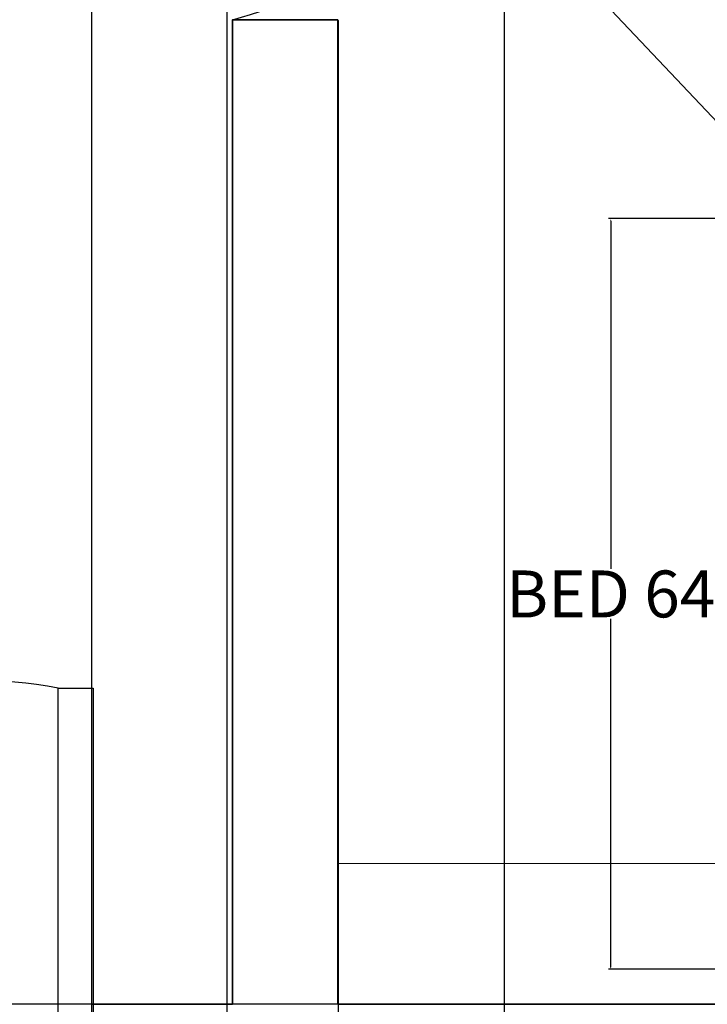
# Model space of a CAD drawing. Units: inches. Extents: x 1291 to 2095, y 532 to 1090.
# Tile 4 of 14: x 1559 to 1618, y 733 to 817. Entities that reach past the tile are written whole.
import ezdxf

# ---------------------------------------------------------------- set-up
doc = ezdxf.new("R2010")
doc.units = ezdxf.units.IN
doc.header["$MEASUREMENT"] = 0
for name, color, linetype, lineweight in [('A-ANNO-DIMS', 2, 'Continuous', 18), ('A-DOOR', 3, 'Continuous', 25), ('A-FLOR-CASE', 9, 'Continuous', 18), ('A-WALL', 7, 'Continuous', 35)]:
    doc.layers.add(name, color=color, linetype=linetype, lineweight=lineweight)
doc.styles.get("Standard").update_dxf_attribs({"font": 'arial.ttf'})
doc.dimstyles.get("Standard").update_dxf_attribs({"dimtxt": 4, "dimasz": 0.18, "dimexe": 0.18, "dimexo": 0.0625, "dimgap": 0.09, "dimtad": 0, "dimtih": 1, "dimtoh": 1, "dimdec": 0, "dimrnd": 6, "dimzin": 0, "dimdsep": 46, "dimlunit": 3, "dimtxsty": 'Standard', "dimcen": 0.09, "dimadec": 0, "dimazin": 0, "dimtfac": 1, "dimtdec": 0, "dimtofl": 0, "dimtmove": 0, "dimatfit": 3, "dimfxl": 1, "dimtolj": 1, "dimtzin": 0, "dimarcsym": 0})

# ---------------------------------------------------------------- blocks, each defined once
blk = doc.blocks.new('*D30')
at = {"layer": 'A-ANNO-DIMS', "color": 0, "lineweight": -2, "transparency": 16777216}
for p, q in [((1618.87, 799.814), (1609.145, 799.814)), ((1609.325, 799.634), (1609.325, 769.922)), ((1609.325, 735.946), (1609.325, 765.658)), ((1618.87, 735.766), (1609.145, 735.766))]:
    blk.add_line(p, q, dxfattribs=at)
at = {"layer": 'A-ANNO-DIMS', "color": 0, "transparency": 16777216}
for points in [[(1609.295, 799.634), (1609.355, 799.634), (1609.325, 799.814)], [(1609.295, 735.946), (1609.355, 735.946), (1609.325, 735.766)]]:
    blk.add_solid(points, dxfattribs=at)
at = {"layer": 'Defpoints', "color": 0, "transparency": 16777216}
for p in [(1618.932, 799.814), (1609.325, 735.766), (1618.932, 735.766)]:
    blk.add_point(p, dxfattribs=at)
at = {"layer": 'A-ANNO-DIMS', "color": 0, "transparency": 16777216, "insert": (1609.325, 767.79), "char_height": 4, "attachment_point": 5}
blk.add_mtext('\\A1;BED 64', dxfattribs=at)
blk = doc.blocks.new('*D44')
at = {"layer": 'A-ANNO-DIMS', "color": 0, "lineweight": -2, "transparency": 16777216}
for p, q in [((1343.074, 579.843), (1343.074, 1087.16)), ((1343.254, 1086.98), (1451.423, 1086.98)), ((1576.431, 1086.98), (1468.261, 1086.98)), ((1576.611, 579.843), (1576.611, 1087.16))]:
    blk.add_line(p, q, dxfattribs=at)
at = {"layer": 'A-ANNO-DIMS', "color": 0, "transparency": 16777216}
for points in [[(1343.254, 1087.01), (1343.254, 1086.95), (1343.074, 1086.98)], [(1576.431, 1087.01), (1576.431, 1086.95), (1576.611, 1086.98)]]:
    blk.add_solid(points, dxfattribs=at)
at = {"layer": 'Defpoints', "color": 0, "transparency": 16777216}
for p in [(1576.611, 1086.98), (1343.074, 579.78), (1576.611, 579.78)]:
    blk.add_point(p, dxfattribs=at)
at = {"layer": 'A-ANNO-DIMS', "color": 0, "transparency": 16777216, "insert": (1459.842, 1086.98), "char_height": 4, "attachment_point": 5}
blk.add_mtext('\\A1;233.54', dxfattribs=at)
blk = doc.blocks.new('*D46')
at = {"layer": 'A-ANNO-DIMS', "color": 0, "lineweight": -2, "transparency": 16777216}
for p, q in [((1600.27, 579.843), (1600.27, 1087.16)), ((1600.45, 1086.98), (1636.471, 1086.98)), ((1685.404, 1086.98), (1649.383, 1086.98)), ((1685.584, 579.843), (1685.584, 1087.16))]:
    blk.add_line(p, q, dxfattribs=at)
at = {"layer": 'A-ANNO-DIMS', "color": 0, "transparency": 16777216}
for points in [[(1600.45, 1087.01), (1600.45, 1086.95), (1600.27, 1086.98)], [(1685.404, 1087.01), (1685.404, 1086.95), (1685.584, 1086.98)]]:
    blk.add_solid(points, dxfattribs=at)
at = {"layer": 'Defpoints', "color": 0, "transparency": 16777216}
for p in [(1685.584, 1086.98), (1600.27, 579.78), (1685.584, 579.78)]:
    blk.add_point(p, dxfattribs=at)
at = {"layer": 'A-ANNO-DIMS', "color": 0, "transparency": 16777216, "insert": (1642.927, 1086.98), "char_height": 4, "attachment_point": 5}
blk.add_mtext('\\A1;85.31', dxfattribs=at)
blk = doc.blocks.new('*D49')
at = {"layer": 'A-ANNO-DIMS', "color": 0, "lineweight": -2, "transparency": 16777216}
for p, q in [((1694.074, 852.718), (1694.074, 534.4)), ((1586.074, 816.718), (1586.074, 534.4)), ((1586.254, 534.58), (1635.749, 534.58)), ((1693.894, 534.58), (1644.398, 534.58))]:
    blk.add_line(p, q, dxfattribs=at)
at = {"layer": 'A-ANNO-DIMS', "color": 0, "transparency": 16777216}
for points in [[(1586.254, 534.61), (1586.254, 534.55), (1586.074, 534.58)], [(1693.894, 534.61), (1693.894, 534.55), (1694.074, 534.58)]]:
    blk.add_solid(points, dxfattribs=at)
at = {"layer": 'Defpoints', "color": 0, "transparency": 16777216}
for p in [(1694.074, 852.78), (1586.074, 816.78), (1694.074, 534.58)]:
    blk.add_point(p, dxfattribs=at)
at = {"layer": 'A-ANNO-DIMS', "color": 0, "transparency": 16777216, "insert": (1640.074, 534.58), "char_height": 4, "attachment_point": 5}
blk.add_mtext('\\A1;108', dxfattribs=at)
blk = doc.blocks.new('*D51')
at = {"layer": 'A-ANNO-DIMS', "color": 0, "lineweight": -2, "transparency": 16777216}
for p, q in [((1820.011, 852.78), (1297.694, 852.78)), ((1297.874, 852.6), (1297.874, 794.913)), ((1297.874, 732.96), (1297.874, 790.648)), ((1811.011, 732.78), (1297.694, 732.78))]:
    blk.add_line(p, q, dxfattribs=at)
at = {"layer": 'A-ANNO-DIMS', "color": 0, "transparency": 16777216}
for points in [[(1297.844, 852.6), (1297.904, 852.6), (1297.874, 852.78)], [(1297.844, 732.96), (1297.904, 732.96), (1297.874, 732.78)]]:
    blk.add_solid(points, dxfattribs=at)
at = {"layer": 'Defpoints', "color": 0, "transparency": 16777216}
for p in [(1297.874, 852.78), (1820.074, 852.78), (1811.074, 732.78)]:
    blk.add_point(p, dxfattribs=at)
at = {"layer": 'A-ANNO-DIMS', "color": 0, "transparency": 16777216, "insert": (1297.874, 792.78), "char_height": 4, "attachment_point": 5}
blk.add_mtext('\\A1;120', dxfattribs=at)
blk = doc.blocks.new('*D63')
at = {"layer": 'A-ANNO-DIMS', "color": 0, "lineweight": -2, "transparency": 16777216}
for p, q in [((1529.074, 723.843), (1529.074, 1087.16)), ((1529.254, 1086.98), (1544.121, 1086.98)), ((1564.894, 1086.98), (1550.026, 1086.98)), ((1565.074, 723.843), (1565.074, 1087.16))]:
    blk.add_line(p, q, dxfattribs=at)
at = {"layer": 'A-ANNO-DIMS', "color": 0, "transparency": 16777216}
for points in [[(1529.254, 1087.01), (1529.254, 1086.95), (1529.074, 1086.98)], [(1564.894, 1087.01), (1564.894, 1086.95), (1565.074, 1086.98)]]:
    blk.add_solid(points, dxfattribs=at)
at = {"layer": 'Defpoints', "color": 0, "transparency": 16777216}
for p in [(1565.074, 1086.98), (1529.074, 723.78), (1565.074, 723.78)]:
    blk.add_point(p, dxfattribs=at)
at = {"layer": 'A-ANNO-DIMS', "color": 0, "transparency": 16777216, "insert": (1547.074, 1086.98), "char_height": 4, "attachment_point": 5}
blk.add_mtext('\\A1;36', dxfattribs=at)
blk = doc.blocks.new('*D85')
at = {"layer": 'A-ANNO-DIMS', "color": 0, "lineweight": -2, "transparency": 16777216}
for p, q in [((1564.052, 865.509), (1564.232, 865.509)), ((1564.142, 865.419), (1564.142, 865.599)), ((1619.506, 806.844), (1598.868, 828.713)), ((1619.686, 806.844), (1619.506, 806.844))]:
    blk.add_line(p, q, dxfattribs=at)
at = {"layer": 'A-ANNO-DIMS', "color": 0, "transparency": 16777216}
blk.add_solid([(1598.89, 828.733), (1598.846, 828.692), (1598.744, 828.844)], dxfattribs=at)
at = {"layer": 'Defpoints', "color": 0, "transparency": 16777216}
for p in [(1564.142, 865.509), (1598.744, 828.844)]:
    blk.add_point(p, dxfattribs=at)
at = {"layer": 'A-ANNO-DIMS', "color": 0, "transparency": 16777216, "insert": (1628.419, 806.844), "char_height": 4, "attachment_point": 5}
blk.add_mtext('\\A1;R50.42', dxfattribs=at)

msp = doc.modelspace()

# ---------------------------------------------------------------- linework, layer by layer
at = {"layer": 'A-DOOR'}
msp.add_lwpolyline([(1562.2125, 759.7536), (1565.2125, 759.7536), (1565.2125, 723.7536), (1562.2125, 723.7536)], close=True, dxfattribs=at)
for centre, radius, start, end in [((1564.1416, 865.5092), 50.4156, 284.862859, 341.821238), ((1556.5498, 731.7195), 28.6002, 78.580328, 196.116311)]:
    msp.add_arc(centre, radius, start, end, dxfattribs=at)
at = {"layer": 'A-FLOR-CASE'}
msp.add_line((1586.0735, 744.7804), (1618.932, 744.7804), dxfattribs=at)
at = {"layer": 'A-WALL'}
for p, q in [((1577.0735, 732.7804), (1577.0735, 816.7804)), ((1586.0735, 816.7804), (1577.0735, 816.7804)), ((1586.0735, 732.7804), (1586.0735, 816.7804)), ((1565.0735, 732.7804), (1577.0735, 732.7804)), ((1586.0735, 732.7804), (1694.0735, 732.7804))]:
    msp.add_line(p, q, dxfattribs=at)

# ---------------------------------------------------------------- dimensions: what is measured, and where the dimension line sits
at = {"layer": 'A-ANNO-DIMS'}
for base, p1, p2, override, picture, middle in [((1576.6107, 1086.9804), (1343.0735, 579.7804), (1576.6107, 579.7804), {"dimdec": 2, "dimlfac": 1, "dimrnd": 0, "dimzin": 0, "dimdsep": 46, "dimlunit": 2}, '*D44', (1459.8421, 1086.9804)), ((1565.0735, 1086.9804), (1529.0735, 723.7804), (1565.0735, 723.7804), {"dimdec": 0, "dimlfac": 1, "dimrnd": 0, "dimzin": 0, "dimdsep": 46, "dimlunit": 2}, '*D63', (1547.0735, 1086.9804)), ((1685.5842, 1086.9804), (1600.2697, 579.7804), (1685.5842, 579.7804), {"dimdec": 2, "dimlfac": 1, "dimrnd": 0, "dimzin": 0, "dimdsep": 46, "dimlunit": 2}, '*D46', (1642.927, 1086.9804)), ((1694.0735, 534.5804), (1586.0735, 816.7804), (1694.0735, 852.7804), {"dimdec": 0, "dimlfac": 1, "dimrnd": 0, "dimzin": 0, "dimdsep": 46, "dimlunit": 2}, '*D49', (1640.0735, 534.5804))]:
    dim = msp.add_linear_dim(base=base, p1=p1, p2=p2, dimstyle='Standard', override=override, dxfattribs=at)
    dim.commit()
    dim.dimension.update_dxf_attribs({"geometry": picture, "text_midpoint": middle})
dim = msp.add_radius_dim(center=(1564.1416, 865.5092), mpoint=(1598.7445, 828.8435), dimstyle='Standard', override={"dimdec": 2, "dimlfac": 1, "dimrnd": 0, "dimzin": 0, "dimdsep": 46, "dimlunit": 2}, dxfattribs=at)
dim.commit()
dim.dimension.update_dxf_attribs({"geometry": '*D85', "text_midpoint": (1628.4187, 806.8441), "dimtype": 164})
dim = msp.add_linear_dim(base=(1297.8735, 852.7804), p1=(1811.0735, 732.7804), p2=(1820.0735, 852.7804), angle=90, dimstyle='Standard', override={"dimdec": 0, "dimlfac": 1, "dimrnd": 0, "dimzin": 0, "dimdsep": 46, "dimlunit": 2}, dxfattribs=at)
dim.commit()
dim.dimension.update_dxf_attribs({"geometry": '*D51', "text_midpoint": (1297.8735, 792.7804)})
dim = msp.add_linear_dim(base=(1609.3247, 735.7658), p1=(1618.932, 799.8143), p2=(1618.932, 735.7658), angle=270, text='BED <>', dimstyle='Standard', override={"dimdec": 0, "dimlfac": 1, "dimrnd": 0, "dimzin": 0, "dimdsep": 46, "dimlunit": 2}, dxfattribs=at)
dim.commit()
dim.dimension.update_dxf_attribs({"geometry": '*D30', "text_midpoint": (1609.3247, 767.79)})

doc.saveas('drawing.dxf')
